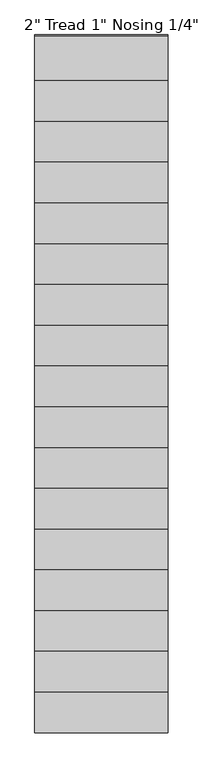
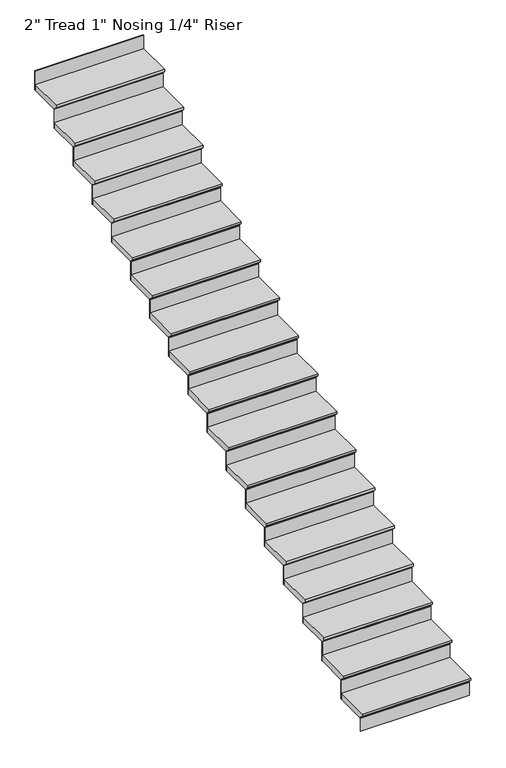
"""IFC4 building model written with IfcOpenShell, lengths in millimetres: stair flight geometry."""

from ifc_helpers import new_model, si_unit, frame, origin, place, context, project, spatial, polyline, outline, extrude, source, transform, mapped, element, save


def stair_flight_dba1ebb1(model_context):
    return source(origin(), model_context, "Body", "SweptSolid", [
        extrude(outline(polyline([(2020.7325341, 474.1333333), (2325.5325341, 474.1333333), (2325.5325341, 423.3333333), (2046.1325341, 423.3333333), (2046.1325341, 429.6833333), (2020.7325341, 455.0833333), (2020.7325341, 474.1333333)])), frame((-5721.5875748, 0.0, 0.0), z_axis=(1.0, 0.0, 0.0), x_axis=(0.0, 1.0, 0.0)), (0.0, 0.0, 1.0), 914.4),
        extrude(outline(polyline([(-4807.1875748, 2052.4825341), (-4807.1875748, 2046.1325341), (-5721.5875748, 2046.1325341), (-5721.5875748, 2052.4825341), (-4807.1875748, 2052.4825341)])), frame((0.0, 0.0, 304.8), z_axis=(0.0, 0.0, 1.0), x_axis=(1.0, 0.0, 0.0)), (0.0, 0.0, 1.0), 118.5333333),
        extrude(outline(polyline([(-4807.1875748, 2331.8825341), (-4807.1875748, 2325.5325341), (-5721.5875748, 2325.5325341), (-5721.5875748, 2331.8825341), (-4807.1875748, 2331.8825341)])), frame((0.0, 0.0, 423.3333333), z_axis=(0.0, 0.0, 1.0), x_axis=(1.0, 0.0, 0.0)), (0.0, 0.0, 1.0), 169.3333333),
        extrude(outline(polyline([(2300.1325341, 643.4666667), (2604.9325341, 643.4666667), (2604.9325341, 592.6666667), (2325.5325341, 592.6666667), (2325.5325341, 599.0166667), (2300.1325341, 624.4166667), (2300.1325341, 643.4666667)])), frame((-5721.5875748, 0.0, 0.0), z_axis=(1.0, 0.0, 0.0), x_axis=(0.0, 1.0, 0.0)), (0.0, 0.0, 1.0), 914.4),
        extrude(outline(polyline([(-4807.1875748, 2611.2825341), (-4807.1875748, 2604.9325341), (-5721.5875748, 2604.9325341), (-5721.5875748, 2611.2825341), (-4807.1875748, 2611.2825341)])), frame((0.0, 0.0, 592.6666667), z_axis=(0.0, 0.0, 1.0), x_axis=(1.0, 0.0, 0.0)), (0.0, 0.0, 1.0), 169.3333333),
        extrude(outline(polyline([(2579.5325341, 812.8), (2884.3325341, 812.8), (2884.3325341, 762.0), (2604.9325341, 762.0), (2604.9325341, 768.35), (2579.5325341, 793.75), (2579.5325341, 812.8)])), frame((-5721.5875748, 0.0, 0.0), z_axis=(1.0, 0.0, 0.0), x_axis=(0.0, 1.0, 0.0)), (0.0, 0.0, 1.0), 914.4),
        extrude(outline(polyline([(-4807.1875748, 2890.6825341), (-4807.1875748, 2884.3325341), (-5721.5875748, 2884.3325341), (-5721.5875748, 2890.6825341), (-4807.1875748, 2890.6825341)])), frame((0.0, 0.0, 762.0), z_axis=(0.0, 0.0, 1.0), x_axis=(1.0, 0.0, 0.0)), (0.0, 0.0, 1.0), 169.3333333),
        extrude(outline(polyline([(2858.9325341, 982.1333333), (3163.7325341, 982.1333333), (3163.7325341, 931.3333333), (2884.3325341, 931.3333333), (2884.3325341, 937.6833333), (2858.9325341, 963.0833333), (2858.9325341, 982.1333333)])), frame((-5721.5875748, 0.0, 0.0), z_axis=(1.0, 0.0, 0.0), x_axis=(0.0, 1.0, 0.0)), (0.0, 0.0, 1.0), 914.4),
        extrude(outline(polyline([(-4807.1875748, 3170.0825341), (-4807.1875748, 3163.7325341), (-5721.5875748, 3163.7325341), (-5721.5875748, 3170.0825341), (-4807.1875748, 3170.0825341)])), frame((0.0, 0.0, 931.3333333), z_axis=(0.0, 0.0, 1.0), x_axis=(1.0, 0.0, 0.0)), (0.0, 0.0, 1.0), 169.3333333),
        extrude(outline(polyline([(3138.3325341, 1151.4666667), (3443.1325341, 1151.4666667), (3443.1325341, 1100.6666667), (3163.7325341, 1100.6666667), (3163.7325341, 1107.0166667), (3138.3325341, 1132.4166667), (3138.3325341, 1151.4666667)])), frame((-5721.5875748, 0.0, 0.0), z_axis=(1.0, 0.0, 0.0), x_axis=(0.0, 1.0, 0.0)), (0.0, 0.0, 1.0), 914.4),
        extrude(outline(polyline([(-4807.1875748, 3449.4825341), (-4807.1875748, 3443.1325341), (-5721.5875748, 3443.1325341), (-5721.5875748, 3449.4825341), (-4807.1875748, 3449.4825341)])), frame((0.0, 0.0, 1100.6666667), z_axis=(0.0, 0.0, 1.0), x_axis=(1.0, 0.0, 0.0)), (0.0, 0.0, 1.0), 169.3333333),
        extrude(outline(polyline([(3417.7325341, 1320.8), (3722.5325341, 1320.8), (3722.5325341, 1270.0), (3443.1325341, 1270.0), (3443.1325341, 1276.35), (3417.7325341, 1301.75), (3417.7325341, 1320.8)])), frame((-5721.5875748, 0.0, 0.0), z_axis=(1.0, 0.0, 0.0), x_axis=(0.0, 1.0, 0.0)), (0.0, 0.0, 1.0), 914.4),
        extrude(outline(polyline([(-4807.1875748, 3728.8825341), (-4807.1875748, 3722.5325341), (-5721.5875748, 3722.5325341), (-5721.5875748, 3728.8825341), (-4807.1875748, 3728.8825341)])), frame((0.0, 0.0, 1270.0), z_axis=(0.0, 0.0, 1.0), x_axis=(1.0, 0.0, 0.0)), (0.0, 0.0, 1.0), 169.3333333),
        extrude(outline(polyline([(3697.1325341, 1490.1333333), (4001.9325341, 1490.1333333), (4001.9325341, 1439.3333333), (3722.5325341, 1439.3333333), (3722.5325341, 1445.6833333), (3697.1325341, 1471.0833333), (3697.1325341, 1490.1333333)])), frame((-5721.5875748, 0.0, 0.0), z_axis=(1.0, 0.0, 0.0), x_axis=(0.0, 1.0, 0.0)), (0.0, 0.0, 1.0), 914.4),
        extrude(outline(polyline([(-4807.1875748, 4008.2825341), (-4807.1875748, 4001.9325341), (-5721.5875748, 4001.9325341), (-5721.5875748, 4008.2825341), (-4807.1875748, 4008.2825341)])), frame((0.0, 0.0, 1439.3333333), z_axis=(0.0, 0.0, 1.0), x_axis=(1.0, 0.0, 0.0)), (0.0, 0.0, 1.0), 169.3333333),
        extrude(outline(polyline([(3976.5325341, 1659.4666667), (4281.3325341, 1659.4666667), (4281.3325341, 1608.6666667), (4001.9325341, 1608.6666667), (4001.9325341, 1615.0166667), (3976.5325341, 1640.4166667), (3976.5325341, 1659.4666667)])), frame((-5721.5875748, 0.0, 0.0), z_axis=(1.0, 0.0, 0.0), x_axis=(0.0, 1.0, 0.0)), (0.0, 0.0, 1.0), 914.4),
        extrude(outline(polyline([(-4807.1875748, 4287.6825341), (-4807.1875748, 4281.3325341), (-5721.5875748, 4281.3325341), (-5721.5875748, 4287.6825341), (-4807.1875748, 4287.6825341)])), frame((0.0, 0.0, 1608.6666667), z_axis=(0.0, 0.0, 1.0), x_axis=(1.0, 0.0, 0.0)), (0.0, 0.0, 1.0), 169.3333333),
        extrude(outline(polyline([(4255.9325341, 1828.8), (4560.7325341, 1828.8), (4560.7325341, 1778.0), (4281.3325341, 1778.0), (4281.3325341, 1784.35), (4255.9325341, 1809.75), (4255.9325341, 1828.8)])), frame((-5721.5875748, 0.0, 0.0), z_axis=(1.0, 0.0, 0.0), x_axis=(0.0, 1.0, 0.0)), (0.0, 0.0, 1.0), 914.4),
        extrude(outline(polyline([(-4807.1875748, 4567.0825341), (-4807.1875748, 4560.7325341), (-5721.5875748, 4560.7325341), (-5721.5875748, 4567.0825341), (-4807.1875748, 4567.0825341)])), frame((0.0, 0.0, 1778.0), z_axis=(0.0, 0.0, 1.0), x_axis=(1.0, 0.0, 0.0)), (0.0, 0.0, 1.0), 169.3333333),
        extrude(outline(polyline([(4535.3325341, 1998.1333333), (4840.1325341, 1998.1333333), (4840.1325341, 1947.3333333), (4560.7325341, 1947.3333333), (4560.7325341, 1953.6833333), (4535.3325341, 1979.0833333), (4535.3325341, 1998.1333333)])), frame((-5721.5875748, 0.0, 0.0), z_axis=(1.0, 0.0, 0.0), x_axis=(0.0, 1.0, 0.0)), (0.0, 0.0, 1.0), 914.4),
        extrude(outline(polyline([(-4807.1875748, 4846.4825341), (-4807.1875748, 4840.1325341), (-5721.5875748, 4840.1325341), (-5721.5875748, 4846.4825341), (-4807.1875748, 4846.4825341)])), frame((0.0, 0.0, 1947.3333333), z_axis=(0.0, 0.0, 1.0), x_axis=(1.0, 0.0, 0.0)), (0.0, 0.0, 1.0), 169.3333333),
        extrude(outline(polyline([(4814.7325341, 2167.4666667), (5119.5325341, 2167.4666667), (5119.5325341, 2116.6666667), (4840.1325341, 2116.6666667), (4840.1325341, 2123.0166667), (4814.7325341, 2148.4166667), (4814.7325341, 2167.4666667)])), frame((-5721.5875748, 0.0, 0.0), z_axis=(1.0, 0.0, 0.0), x_axis=(0.0, 1.0, 0.0)), (0.0, 0.0, 1.0), 914.4),
        extrude(outline(polyline([(-4807.1875748, 5125.8825341), (-4807.1875748, 5119.5325341), (-5721.5875748, 5119.5325341), (-5721.5875748, 5125.8825341), (-4807.1875748, 5125.8825341)])), frame((0.0, 0.0, 2116.6666667), z_axis=(0.0, 0.0, 1.0), x_axis=(1.0, 0.0, 0.0)), (0.0, 0.0, 1.0), 169.3333333),
        extrude(outline(polyline([(5094.1325341, 2336.8), (5398.9325341, 2336.8), (5398.9325341, 2286.0), (5119.5325341, 2286.0), (5119.5325341, 2292.35), (5094.1325341, 2317.75), (5094.1325341, 2336.8)])), frame((-5721.5875748, 0.0, 0.0), z_axis=(1.0, 0.0, 0.0), x_axis=(0.0, 1.0, 0.0)), (0.0, 0.0, 1.0), 914.4),
        extrude(outline(polyline([(-4807.1875748, 5405.2825341), (-4807.1875748, 5398.9325341), (-5721.5875748, 5398.9325341), (-5721.5875748, 5405.2825341), (-4807.1875748, 5405.2825341)])), frame((0.0, 0.0, 2286.0), z_axis=(0.0, 0.0, 1.0), x_axis=(1.0, 0.0, 0.0)), (0.0, 0.0, 1.0), 169.3333333),
        extrude(outline(polyline([(5373.5325341, 2506.1333333), (5678.3325341, 2506.1333333), (5678.3325341, 2455.3333333), (5398.9325341, 2455.3333333), (5398.9325341, 2461.6833333), (5373.5325341, 2487.0833333), (5373.5325341, 2506.1333333)])), frame((-5721.5875748, 0.0, 0.0), z_axis=(1.0, 0.0, 0.0), x_axis=(0.0, 1.0, 0.0)), (0.0, 0.0, 1.0), 914.4),
        extrude(outline(polyline([(-4807.1875748, 5684.6825341), (-4807.1875748, 5678.3325341), (-5721.5875748, 5678.3325341), (-5721.5875748, 5684.6825341), (-4807.1875748, 5684.6825341)])), frame((0.0, 0.0, 2455.3333333), z_axis=(0.0, 0.0, 1.0), x_axis=(1.0, 0.0, 0.0)), (0.0, 0.0, 1.0), 169.3333333),
        extrude(outline(polyline([(5652.9325341, 2675.4666667), (5957.7325341, 2675.4666667), (5957.7325341, 2624.6666667), (5678.3325341, 2624.6666667), (5678.3325341, 2631.0166667), (5652.9325341, 2656.4166667), (5652.9325341, 2675.4666667)])), frame((-5721.5875748, 0.0, 0.0), z_axis=(1.0, 0.0, 0.0), x_axis=(0.0, 1.0, 0.0)), (0.0, 0.0, 1.0), 914.4),
        extrude(outline(polyline([(-4807.1875748, 5964.0825341), (-4807.1875748, 5957.7325341), (-5721.5875748, 5957.7325341), (-5721.5875748, 5964.0825341), (-4807.1875748, 5964.0825341)])), frame((0.0, 0.0, 2624.6666667), z_axis=(0.0, 0.0, 1.0), x_axis=(1.0, 0.0, 0.0)), (0.0, 0.0, 1.0), 169.3333333),
        extrude(outline(polyline([(5932.3325341, 2844.8), (6237.1325341, 2844.8), (6237.1325341, 2794.0), (5957.7325341, 2794.0), (5957.7325341, 2800.35), (5932.3325341, 2825.75), (5932.3325341, 2844.8)])), frame((-5721.5875748, 0.0, 0.0), z_axis=(1.0, 0.0, 0.0), x_axis=(0.0, 1.0, 0.0)), (0.0, 0.0, 1.0), 914.4),
        extrude(outline(polyline([(-4807.1875748, 6243.4825341), (-4807.1875748, 6237.1325341), (-5721.5875748, 6237.1325341), (-5721.5875748, 6243.4825341), (-4807.1875748, 6243.4825341)])), frame((0.0, 0.0, 2794.0), z_axis=(0.0, 0.0, 1.0), x_axis=(1.0, 0.0, 0.0)), (0.0, 0.0, 1.0), 169.3333333),
        extrude(outline(polyline([(6211.7325341, 3014.1333333), (6516.5325341, 3014.1333333), (6516.5325341, 2963.3333333), (6237.1325341, 2963.3333333), (6237.1325341, 2969.6833333), (6211.7325341, 2995.0833333), (6211.7325341, 3014.1333333)])), frame((-5721.5875748, 0.0, 0.0), z_axis=(1.0, 0.0, 0.0), x_axis=(0.0, 1.0, 0.0)), (0.0, 0.0, 1.0), 914.4),
        extrude(outline(polyline([(-4807.1875748, 6522.8825341), (-4807.1875748, 6516.5325341), (-5721.5875748, 6516.5325341), (-5721.5875748, 6522.8825341), (-4807.1875748, 6522.8825341)])), frame((0.0, 0.0, 2963.3333333), z_axis=(0.0, 0.0, 1.0), x_axis=(1.0, 0.0, 0.0)), (0.0, 0.0, 1.0), 169.3333333),
        extrude(outline(polyline([(-4807.1875748, 6802.2825341), (-4807.1875748, 6795.9325341), (-5721.5875748, 6795.9325341), (-5721.5875748, 6802.2825341), (-4807.1875748, 6802.2825341)])), frame((0.0, 0.0, 3132.6666667), z_axis=(0.0, 0.0, 1.0), x_axis=(1.0, 0.0, 0.0)), (0.0, 0.0, 1.0), 169.3333333),
        extrude(outline(polyline([(6491.1325341, 3183.4666667), (6795.9325341, 3183.4666667), (6795.9325341, 3132.6666667), (6516.5325341, 3132.6666667), (6516.5325341, 3139.0166667), (6491.1325341, 3164.4166667), (6491.1325341, 3183.4666667)])), frame((-5721.5875748, 0.0, 0.0), z_axis=(1.0, 0.0, 0.0), x_axis=(0.0, 1.0, 0.0)), (0.0, 0.0, 1.0), 914.4),
    ])


if __name__ == "__main__":
    model = new_model("IFC4")
    model_context = context("Model", 3, world=origin())
    ifc_project = project(units=[si_unit("LENGTHUNIT", "METRE", prefix="MILLI")], contexts=[model_context])
    site = spatial("IfcSite", under=ifc_project)
    building = spatial("IfcBuilding", under=site)
    placement = place(None, origin())
    stair_flight_shape = stair_flight_dba1ebb1(model_context)
    element("IfcStairFlight", 1, ObjectType="2\" Tread 1\" Nosing 1/4\" Riser", at=placement, inside=building, context=model_context, shape_type="MappedRepresentation", body=[
        mapped(stair_flight_shape, transform((0.0, 0.0, 0.0), x_axis=(1.0, 0.0, 0.0), y_axis=(0.0, 1.0, 0.0), z_axis=(0.0, 0.0, 1.0))),
    ])
    save(model, "model.ifc")
